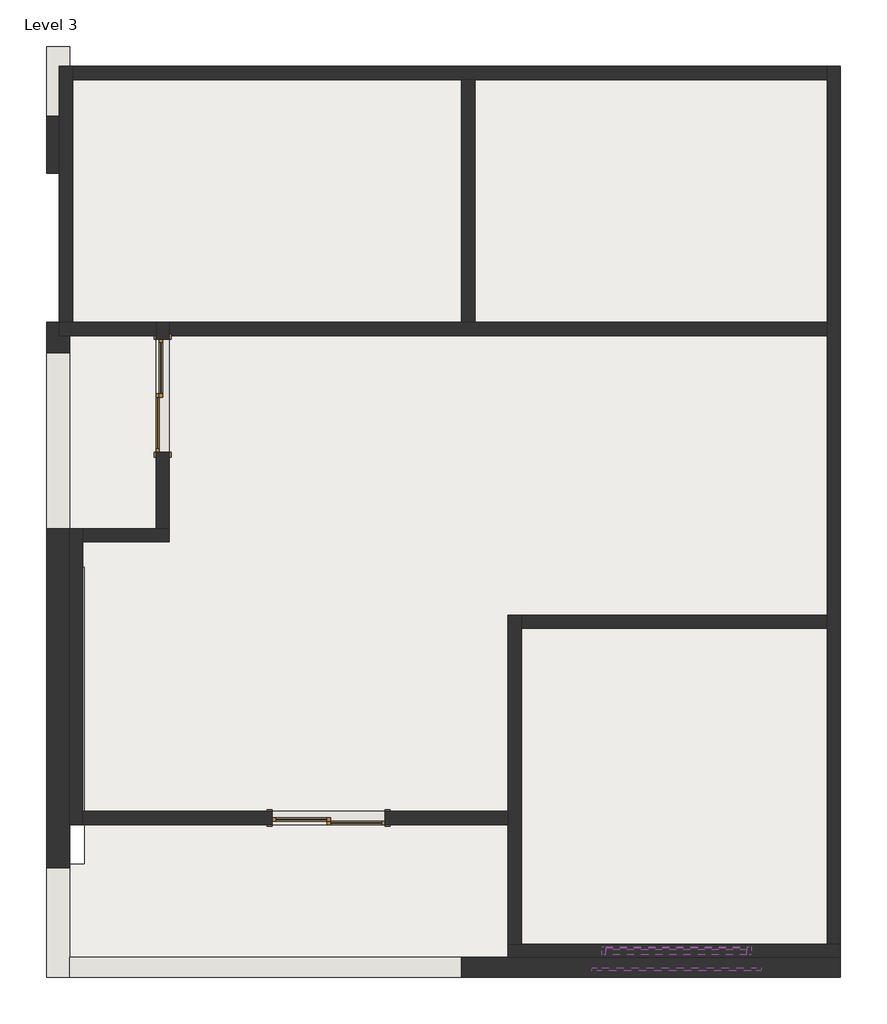
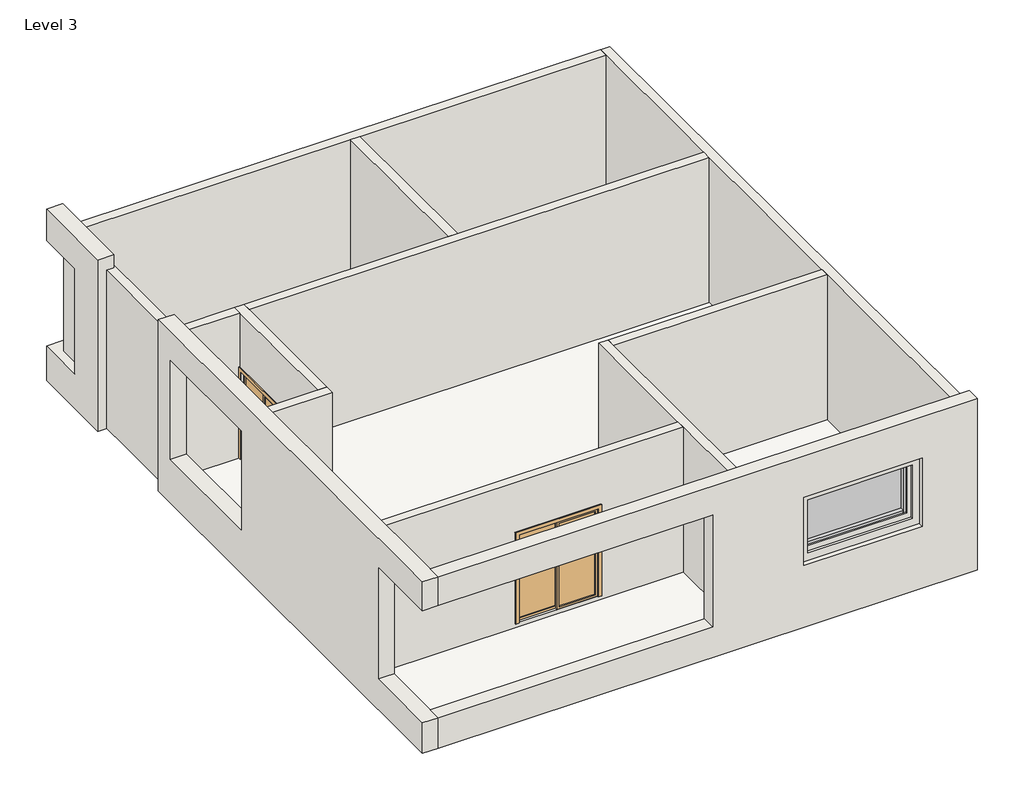
# One storey: 16 walls, 4 members, 2 doors, 1 plate, 1 roof.
"""IFC4 building model written with IfcOpenShell, lengths in millimetres."""

from ifc_helpers import new_model, si_unit, frame, origin, place, context, project, spatial, polyline, outline, extrude, faceted_brep, transform, mapped, element, save
from components import door_076b30e0, member_3a6679d5, member_c08f7e50, system_panel_glazed_5a0db22b, walls_4_walls_1_cdf310b5, walls_5_walls_6_e556a0bb, walls_9_walls_5_51837564

model = new_model("IFC4")

# Units and contexts
model_context = context("Model", 3, world=origin())
ifc_project = project(units=[si_unit("LENGTHUNIT", "METRE", prefix="MILLI")], contexts=[model_context])

# Site, building, storey
site = spatial("IfcSite", under=ifc_project)
building = spatial("IfcBuilding", under=site)
storey = spatial("IfcBuildingStorey", under=building, Name="Level 3", Elevation=7315.2)

# Doors
placement = place(None, origin())
door_shape = door_076b30e0(model_context)
element("IfcDoor", 1, ObjectType="Door-Double-Sliding : 68\" x 80\"", at=placement, inside=storey, context=model_context, shape_type="MappedRepresentation", body=[
    mapped(door_shape, transform((-7311.1727738, 4595.9674246, 7620.0), x_axis=(0.0, 1.0, 0.0), y_axis=(-1.0, 0.0, 0.0), z_axis=(0.0, 0.0, 1.0))),
])
element("IfcDoor", 2, ObjectType="Door-Double-Sliding : 68\" x 80\"", at=placement, inside=storey, context=model_context, shape_type="MappedRepresentation", body=[
    mapped(door_shape, transform((-4898.5436544, -1728.6325754, 7721.6), x_axis=(-1.0, 0.0, 0.0), y_axis=(0.0, -1.0, 0.0), z_axis=(0.0, 0.0, 1.0))),
])

# Members
member_shape = member_3a6679d5(model_context)
element("IfcMember", 3, ObjectType="Rectangular Mullion : 2.5\" x 5\" rectangular", at=placement, inside=storey, context=model_context, shape_type="MappedRepresentation", body=[
    mapped(member_shape, transform((1560.0533085, -3887.6325754, 8918.7422066), x_axis=(1.0, 0.0, 0.0), y_axis=(0.0, -1.0, 0.0), z_axis=(0.0, 0.0, -1.0))),
])
member_2_shape = member_c08f7e50(model_context)
element("IfcMember", 4, ObjectType="Rectangular Mullion : 2.5\" x 5\" rectangular", at=placement, inside=storey, context=model_context, shape_type="MappedRepresentation", body=[
    mapped(member_2_shape, transform((-662.4466915, -3887.6325754, 8918.7422066), x_axis=(0.0, 0.0, -1.0), y_axis=(0.0, -1.0, 0.0), z_axis=(-1.0, 0.0, 0.0))),
])
element("IfcMember", 5, ObjectType="Rectangular Mullion : 2.5\" x 5\" rectangular", at=placement, inside=storey, context=model_context, shape_type="MappedRepresentation", body=[
    mapped(member_2_shape, transform((1496.5533085, -3887.6325754, 10149.624337), x_axis=(0.0, 0.0, 1.0), y_axis=(0.0, -1.0, 0.0), z_axis=(1.0, 0.0, 0.0))),
])
element("IfcMember", 6, ObjectType="Rectangular Mullion : 2.5\" x 5\" rectangular", at=placement, inside=storey, context=model_context, shape_type="MappedRepresentation", body=[
    mapped(member_shape, transform((-725.9466915, -3887.6325754, 10149.624337), x_axis=(-1.0, 0.0, 0.0), y_axis=(0.0, -1.0, 0.0), z_axis=(0.0, 0.0, 1.0))),
])

# Plate
system_panel_glazed_shape = system_panel_glazed_5a0db22b(model_context)
element("IfcPlate", 7, ObjectType="System Panel : Glazed", at=placement, inside=storey, context=model_context, shape_type="MappedRepresentation", body=[
    mapped(system_panel_glazed_shape, transform((417.0533085, -3887.6325754, 8982.2422066), x_axis=(1.0, 0.0, 0.0), y_axis=(0.0, 1.0, 0.0), z_axis=(0.0, 0.0, 1.0))),
])

# Roof
element("IfcRoof", 8, ObjectType="Generic - 12\"", at=placement, inside=storey, context=model_context, shape_type="SweptSolid", body=[
    extrude(outline(polyline([(-8860.5727738, 9472.7674246), (2924.6563456, 9472.7674246), (2924.6563456, -3989.2325754), (-8860.5727738, -3989.2325754), (-8860.5727738, -2566.8325754), (-8631.9727738, -2566.8325754), (-8631.9727738, 1979.7674246), (-8860.5727738, 1979.7674246), (-8860.5727738, 9472.7674246)])), frame((0.0, 0.0, 7315.2), z_axis=(0.0, 0.0, 1.0), x_axis=(1.0, 0.0, 0.0)), (0.0, 0.0, 1.0), 304.8),
])

# Walls
element("IfcWall", 9, ObjectType="Generic - 8\"", at=placement, inside=storey, context=model_context, shape_type="Brep", body=[
    faceted_brep([(2924.6563456, -3786.0325754, 7315.2), (2721.4563456, -3786.0325754, 7315.2), (-1952.1436544, -3786.0325754, 7315.2), (-2155.3436544, -3786.0325754, 7315.2), (-2155.3436544, -3786.0325754, 10972.8), (-1952.1436544, -3786.0325754, 10972.8), (2721.4563456, -3786.0325754, 10972.8), (2924.6563456, -3786.0325754, 10972.8), (1560.0533085, -3786.0325754, 10149.624337), (-725.9466915, -3786.0325754, 10149.624337), (-725.9466915, -3786.0325754, 8918.7422066), (1560.0533085, -3786.0325754, 8918.7422066), (2924.6563456, -3989.2325754, 7315.2), (2924.6563456, -3989.2325754, 10972.8), (-2155.3436544, -3989.2325754, 10972.8), (-2155.3436544, -3989.2325754, 7315.2), (1560.0533085, -3989.2325754, 10149.624337), (1560.0533085, -3989.2325754, 8918.7422066), (-725.9466915, -3989.2325754, 8918.7422066), (-725.9466915, -3989.2325754, 10149.624337)], [[[0, 1, 2, 3, 4, 5, 6, 7], [8, 9, 10, 11]], [[12, 13, 14, 15], [16, 17, 18, 19]], [[4, 3, 15, 14]], [[0, 7, 13, 12]], [[3, 2, 1, 0, 12, 15]], [[7, 6, 5, 4, 14, 13]], [[9, 8, 16, 19]], [[10, 9, 19, 18]], [[11, 10, 18, 17]], [[8, 11, 17, 16]]]),
])
element("IfcWall", 10, ObjectType="Generic - 8\"", at=placement, inside=storey, context=model_context, shape_type="Brep", body=[
    faceted_brep([(-1952.1436544, -3786.0325754, 7315.2), (-1952.1436544, 1039.9674246, 7315.2), (-1952.1436544, 1243.1674246, 7315.2), (-1952.1436544, 1243.1674246, 10972.8), (-1952.1436544, 1039.9674246, 10972.8), (-1952.1436544, -3786.0325754, 10972.8), (-2155.3436544, -3786.0325754, 7315.2), (-2155.3436544, -3786.0325754, 10972.8), (-2155.3436544, -1957.2325754, 10972.8), (-2155.3436544, -1754.0325754, 10972.8), (-2155.3436544, 1243.1674246, 10972.8), (-2155.3436544, 1243.1674246, 7315.2), (-2155.3436544, -1754.0325754, 7315.2), (-2155.3436544, -1957.2325754, 7315.2)], [[[0, 1, 2, 3, 4, 5]], [[6, 7, 8, 9, 10, 11, 12, 13]], [[2, 1, 0, 6, 13, 12, 11]], [[5, 4, 3, 10, 9, 8, 7]], [[0, 5, 7, 6]], [[3, 2, 11, 10]]]),
])
element("IfcWall", 11, ObjectType="Generic - 8\"", at=placement, inside=storey, context=model_context, shape_type="SweptSolid", body=[
    extrude(outline(polyline([(2716.475018, 1039.9674246), (-1952.1436544, 1039.9674246), (-1952.1436544, 1243.1674246), (2716.475018, 1243.1674246), (2716.475018, 1039.9674246)])), frame((0.0, 0.0, 7315.2), z_axis=(0.0, 0.0, 1.0), x_axis=(1.0, 0.0, 0.0)), (0.0, 0.0, 1.0), 3657.6),
])
element("IfcWall", 12, ObjectType="Generic - 8\"", at=placement, inside=storey, context=model_context, shape_type="SweptSolid", body=[
    extrude(outline(polyline([(2924.6563456, 9625.1674246), (2924.6563456, -3786.0325754), (2721.4563456, -3786.0325754), (2721.4563456, 9625.1674246), (2924.6563456, 9625.1674246)])), frame((0.0, 0.0, 7315.2), z_axis=(0.0, 0.0, 1.0), x_axis=(1.0, 0.0, 0.0)), (0.0, 0.0, 1.0), 3657.6),
])
element("IfcWall", 13, ObjectType="Generic - 8\"", at=placement, inside=storey, context=model_context, shape_type="Brep", body=[
    faceted_brep([(-8657.3727738, -1957.2325754, 7315.2), (-8657.3727738, -1754.0325754, 7315.2), (-8657.3727738, 2360.7674246, 7315.2), (-8657.3727738, 2563.9674246, 7315.2), (-8657.3727738, 2563.9674246, 10972.8), (-8657.3727738, 2360.7674246, 10972.8), (-8657.3727738, -1754.0325754, 10972.8), (-8657.3727738, -1957.2325754, 10972.8), (-8860.5727738, -1957.2325754, 7315.2), (-8860.5727738, -1957.2325754, 10972.8), (-8860.5727738, 2563.9674246, 10972.8), (-8860.5727738, 2563.9674246, 7315.2)], [[[0, 1, 2, 3, 4, 5, 6, 7]], [[8, 9, 10, 11]], [[3, 2, 1, 0, 8, 11]], [[7, 6, 5, 4, 10, 9]], [[4, 3, 11, 10]], [[0, 7, 9, 8]]]),
])
element("IfcWall", 14, ObjectType="Generic - 8\"", at=placement, inside=storey, context=model_context, shape_type="Brep", body=[
    faceted_brep([(-8657.3727738, 2360.7674246, 7315.2), (-7336.5727738, 2360.7674246, 7315.2), (-7336.5727738, 2360.7674246, 10972.8), (-8657.3727738, 2360.7674246, 10972.8), (-8657.3727738, 2563.9674246, 7315.2), (-8657.3727738, 2563.9674246, 10972.8), (-7539.7727738, 2563.9674246, 10972.8), (-7336.5727738, 2563.9674246, 10972.8), (-7336.5727738, 2563.9674246, 7315.2), (-7539.7727738, 2563.9674246, 7315.2)], [[[0, 1, 2, 3]], [[4, 5, 6, 7, 8, 9]], [[1, 0, 4, 9, 8]], [[3, 2, 7, 6, 5]], [[0, 3, 5, 4]], [[2, 1, 8, 7]]]),
])
element("IfcWall", 15, ObjectType="Generic - 8\"", at=placement, inside=storey, context=model_context, shape_type="Brep", body=[
    faceted_brep([(-7336.5727738, 2563.9674246, 7315.2), (-7336.5727738, 5510.3674246, 7315.2), (-7336.5727738, 5713.5674246, 7315.2), (-7336.5727738, 5713.5674246, 10972.8), (-7336.5727738, 5510.3674246, 10972.8), (-7336.5727738, 2563.9674246, 10972.8), (-7336.5727738, 3732.3674246, 9652.0), (-7336.5727738, 5459.5674246, 9652.0), (-7336.5727738, 5459.5674246, 7620.0), (-7336.5727738, 3732.3674246, 7620.0), (-7539.7727738, 2563.9674246, 7315.2), (-7539.7727738, 2563.9674246, 10972.8), (-7539.7727738, 5510.3674246, 10972.8), (-7539.7727738, 5713.5674246, 10972.8), (-7539.7727738, 5713.5674246, 7315.2), (-7539.7727738, 5510.3674246, 7315.2), (-7539.7727738, 3732.3674246, 9652.0), (-7539.7727738, 3732.3674246, 7620.0), (-7539.7727738, 5459.5674246, 7620.0), (-7539.7727738, 5459.5674246, 9652.0)], [[[0, 1, 2, 3, 4, 5], [6, 7, 8, 9]], [[10, 11, 12, 13, 14, 15], [16, 17, 18, 19]], [[2, 1, 0, 10, 15, 14]], [[5, 4, 3, 13, 12, 11]], [[0, 5, 11, 10]], [[3, 2, 14, 13]], [[17, 16, 6, 9]], [[18, 17, 9, 8]], [[19, 18, 8, 7]], [[16, 19, 7, 6]]]),
])
element("IfcWall", 16, ObjectType="Generic - 8\"", at=placement, inside=storey, context=model_context, shape_type="Brep", body=[
    faceted_brep([(-7539.7727738, 5713.5674246, 7315.2), (-8815.124982, 5713.5674246, 7315.2), (-9018.324982, 5713.5674246, 7315.2), (-9018.324982, 5713.5674246, 10972.8), (-8815.124982, 5713.5674246, 10972.8), (-7539.7727738, 5713.5674246, 10972.8), (-7539.7727738, 5510.3674246, 7315.2), (-7539.7727738, 5510.3674246, 10972.8), (-9018.324982, 5510.3674246, 10972.8), (-9018.324982, 5510.3674246, 7315.2)], [[[0, 1, 2, 3, 4, 5]], [[6, 7, 8, 9]], [[2, 1, 0, 6, 9]], [[5, 4, 3, 8, 7]], [[0, 5, 7, 6]], [[3, 2, 9, 8]]]),
])
element("IfcWall", 17, ObjectType="Generic - 8\"", at=placement, inside=storey, context=model_context, shape_type="Brep", body=[
    faceted_brep([(-8815.124982, 5713.5674246, 7315.2), (-8815.124982, 9421.9674246, 7315.2), (-8815.124982, 9625.1674246, 7315.2), (-8815.124982, 9625.1674246, 10972.8), (-8815.124982, 9421.9674246, 10972.8), (-8815.124982, 5713.5674246, 10972.8), (-9018.324982, 5713.5674246, 7315.2), (-9018.324982, 5713.5674246, 10972.8), (-9018.324982, 9625.1674246, 10972.8), (-9018.324982, 9625.1674246, 7315.2)], [[[0, 1, 2, 3, 4, 5]], [[6, 7, 8, 9]], [[2, 1, 0, 6, 9]], [[5, 4, 3, 8, 7]], [[0, 5, 7, 6]], [[3, 2, 9, 8]]]),
])
element("IfcWall", 18, ObjectType="Generic - 8\"", at=placement, inside=storey, context=model_context, shape_type="Brep", body=[
    faceted_brep([(-8815.124982, 9421.9674246, 7315.2), (-2866.5436544, 9421.9674246, 7315.2), (-2663.3436544, 9421.9674246, 7315.2), (2716.475018, 9421.9674246, 7315.2), (2716.475018, 9421.9674246, 10972.8), (-2663.3436544, 9421.9674246, 10972.8), (-2866.5436544, 9421.9674246, 10972.8), (-8815.124982, 9421.9674246, 10972.8), (-8815.124982, 9625.1674246, 7315.2), (-8815.124982, 9625.1674246, 10972.8), (2716.475018, 9625.1674246, 10972.8), (2716.475018, 9625.1674246, 7315.2)], [[[0, 1, 2, 3, 4, 5, 6, 7]], [[8, 9, 10, 11]], [[3, 2, 1, 0, 8, 11]], [[4, 3, 11, 10]], [[7, 6, 5, 4, 10, 9]], [[0, 7, 9, 8]]]),
])
element("IfcWall", 19, ObjectType="Generic - 8\"", at=placement, inside=storey, context=model_context, shape_type="Brep", body=[
    faceted_brep([(-7336.5727738, 5510.3674246, 7315.2), (2716.475018, 5510.3674246, 7315.2), (2716.475018, 5510.3674246, 10972.8), (-7336.5727738, 5510.3674246, 10972.8), (-7336.5727738, 5713.5674246, 7315.2), (-7336.5727738, 5713.5674246, 10972.8), (-2866.5436544, 5713.5674246, 10972.8), (-2663.3436544, 5713.5674246, 10972.8), (2716.475018, 5713.5674246, 10972.8), (2716.475018, 5713.5674246, 7315.2), (-2663.3436544, 5713.5674246, 7315.2), (-2866.5436544, 5713.5674246, 7315.2)], [[[0, 1, 2, 3]], [[4, 5, 6, 7, 8, 9, 10, 11]], [[1, 0, 4, 11, 10, 9]], [[2, 1, 9, 8]], [[3, 2, 8, 7, 6, 5]], [[0, 3, 5, 4]]]),
])
element("IfcWall", 20, ObjectType="Generic - 8\"", at=placement, inside=storey, context=model_context, shape_type="SweptSolid", body=[
    extrude(outline(polyline([(-2663.3436544, 9421.9674246), (-2663.3436544, 5713.5674246), (-2866.5436544, 5713.5674246), (-2866.5436544, 9421.9674246), (-2663.3436544, 9421.9674246)])), frame((0.0, 0.0, 7315.2), z_axis=(0.0, 0.0, 1.0), x_axis=(1.0, 0.0, 0.0)), (0.0, 0.0, 1.0), 3657.6),
])
element("IfcWall", 21, ObjectType="Generic - 8\"", at=placement, inside=storey, context=model_context, shape_type="SweptSolid", body=[
    extrude(outline(polyline([(7315.2, -8657.3727738), (7315.2, -2155.3436544), (10972.8, -2155.3436544), (10972.8, -8657.3727738), (7315.2, -8657.3727738)]), holes=[polyline([(9753.6, -4034.9436544), (7721.6, -4034.9436544), (7721.6, -5762.1436544), (9753.6, -5762.1436544), (9753.6, -4034.9436544)])]), frame((0.0, -1957.2325754, 0.0), z_axis=(0.0, 1.0, 0.0), x_axis=(0.0, 0.0, 1.0)), (0.0, 0.0, 1.0), 203.2),
])
walls_4_walls_1_shape = walls_4_walls_1_cdf310b5(model_context)
element("IfcWall", 22, ObjectType="Walls 4 : Walls 1", at=placement, inside=storey, context=model_context, shape_type="MappedRepresentation", body=[
    mapped(walls_4_walls_1_shape, transform((0.0, 0.0, 0.0), x_axis=(1.0, 0.0, 0.0), y_axis=(0.0, 1.0, 0.0), z_axis=(0.0, 0.0, 1.0))),
])
walls_5_walls_6_shape = walls_5_walls_6_e556a0bb(model_context)
element("IfcWall", 23, ObjectType="Walls 5 : Walls 6", at=placement, inside=storey, context=model_context, shape_type="MappedRepresentation", body=[
    mapped(walls_5_walls_6_shape, transform((0.0, 0.0, 0.0), x_axis=(1.0, 0.0, 0.0), y_axis=(0.0, 1.0, 0.0), z_axis=(0.0, 0.0, 1.0))),
])
walls_9_walls_5_shape = walls_9_walls_5_51837564(model_context)
element("IfcWall", 24, ObjectType="Walls 9 : Walls 5", at=placement, inside=storey, context=model_context, shape_type="MappedRepresentation", body=[
    mapped(walls_9_walls_5_shape, transform((0.0, 0.0, 0.0), x_axis=(1.0, 0.0, 0.0), y_axis=(0.0, 1.0, 0.0), z_axis=(0.0, 0.0, 1.0))),
])

save(model, "model.ifc")

# Revit data of these elements
# Type "Door-Double-Sliding : 68\" x 80\""
#   Type Mark = "10"
#   Construction Type Id = "opn-d45"
#   Assembly Code = "C1020"
#   Analytic Construction = "Wood frame, double glass door "
#   Thickness = 0' - 2"
#   Thermal Resistance (R) = 1.8150 (h·ft²·°F)/BTU
#   Heat Transfer Coefficient (U) = 0.5510 BTU/(h·ft²·°F)
#   Height = 6' - 8"
#   Rail Width = 0' - 2"
#   Stiles = 0' - 2"
#   Trim Projection Ext = 0' - 1"
#   Trim Projection Int = 0' - 1"
#   Trim Width = 0' - 3"
#   Width = 5' - 8"
#   Define Thermal Properties by = 1
#   Glazing = Glass
#   Panel Material = Wood - Birch - Solid Stained Light Low Gloss
#   Trim Material = Paint - Sienna
#   Visual Light Transmittance = 0
#   Solar Heat Gain Coefficient = 0
#   Function = (empty or 0)
#   Wall Closure = (empty or 0)
# Type "Rectangular Mullion : 2.5\" x 5\" rectangular"
#   built-in parameter 1007304 = 0.416667 (stored number, unit not read)
#   built-in parameter 1007301 = 0.104167 (stored number, unit not read)
#   built-in parameter 1007300 = 0.104167 (stored number, unit not read)
# Type "System Panel : Glazed"
#   Construction Type Id = "GSP4R"
#   Analytic Construction = "1/8 in Pilkington single glazing"
#   Visual Light Transmittance = 0.9
#   Solar Heat Gain Coefficient = 0.86
#   Heat Transfer Coefficient (U) = 1.18115 BTU/(h·ft²·°F)
# Type "Generic - 12\""
#   Assembly Code = "B1020"
#   Layers, outside or top first: 1' - 0" no material (function 1)
# Type "Generic - 8\""
#   Assembly Code = "B2010"
#   Layers, outside or top first: 0' - 8" no material (function 1)
# Elements 1, 2 (IfcDoor, "Door-Double-Sliding : 68\" x 80\"")
#   Phase Created = New Construction
#   Materials on its faces: "Paint - Sienna", "Wood - Birch - Solid Stained Light Low Gloss", "Glass"
# Elements 3, 4, 5, 6 (IfcMember, "Rectangular Mullion : 2.5\" x 5\" rectangular")
#   Phase Created = New Construction
#   Materials on its faces: "Aluminum"
# Element 7 (IfcPlate, "System Panel : Glazed")
#   Phase Created = New Construction
#   Materials on its faces: "Glass"
# Element 8 (IfcRoof, "Generic - 12\"")
#   built-in parameter 1001705 = 25 (stored number, unit not read)
#   built-in parameter 1001710 = 33615
#   Phase Created = New Construction
#   Materials on its faces: "Default Roof"
# Elements 9, 10, 11, 12, 13, 14, 15, 16, 17, 18, 19, 20, 21 (IfcWall, "Generic - 8\"")
#   Top Offset = 0' - 0"
#   Base Offset = 0' - 0"
#   Unconnected Height = 12' - 0"
#   wall height = 12' - 0"
#   Phase Created = New Construction
#   Base Constraint = Level 3
#   Materials on its faces: "Default Wall"
# Element 22 (IfcWall, "Walls 4 : Walls 1")
#   Phase Created = New Construction
#   Materials on its faces: "Default Wall"
# Element 23 (IfcWall, "Walls 5 : Walls 6")
#   Phase Created = New Construction
#   Materials on its faces: "Default Wall"
# Element 24 (IfcWall, "Walls 9 : Walls 5")
#   Phase Created = New Construction
#   Materials on its faces: "Default Wall"
# Materials
#   "Glass": class "Glass", colour RGB 0 128 192, transparency 0.75, Description = "Soda Lime Glass", Cost = 0
#   "Wood - Birch - Solid Stained Light Low Gloss": class "Wood", colour RGB 210 159 95, transparency 0, Cost = 0
#   "Paint - Sienna": colour RGB 118 70 51, transparency 0, Cost = 0
#   "Aluminum": class "Metal", colour RGB 247 247 247, transparency 0, Description = "Aluminum 6061", Cost = 0
#   "Default Roof": colour RGB 88 101 114, transparency 0
#   "Default Wall": colour RGB 128 128 128, transparency 0
